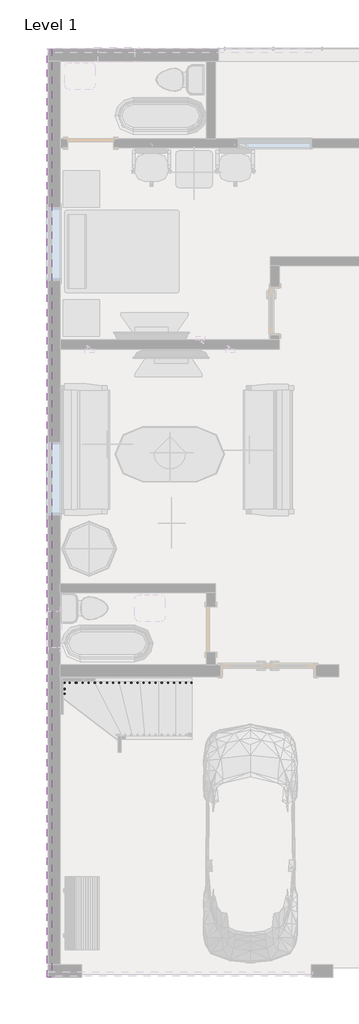
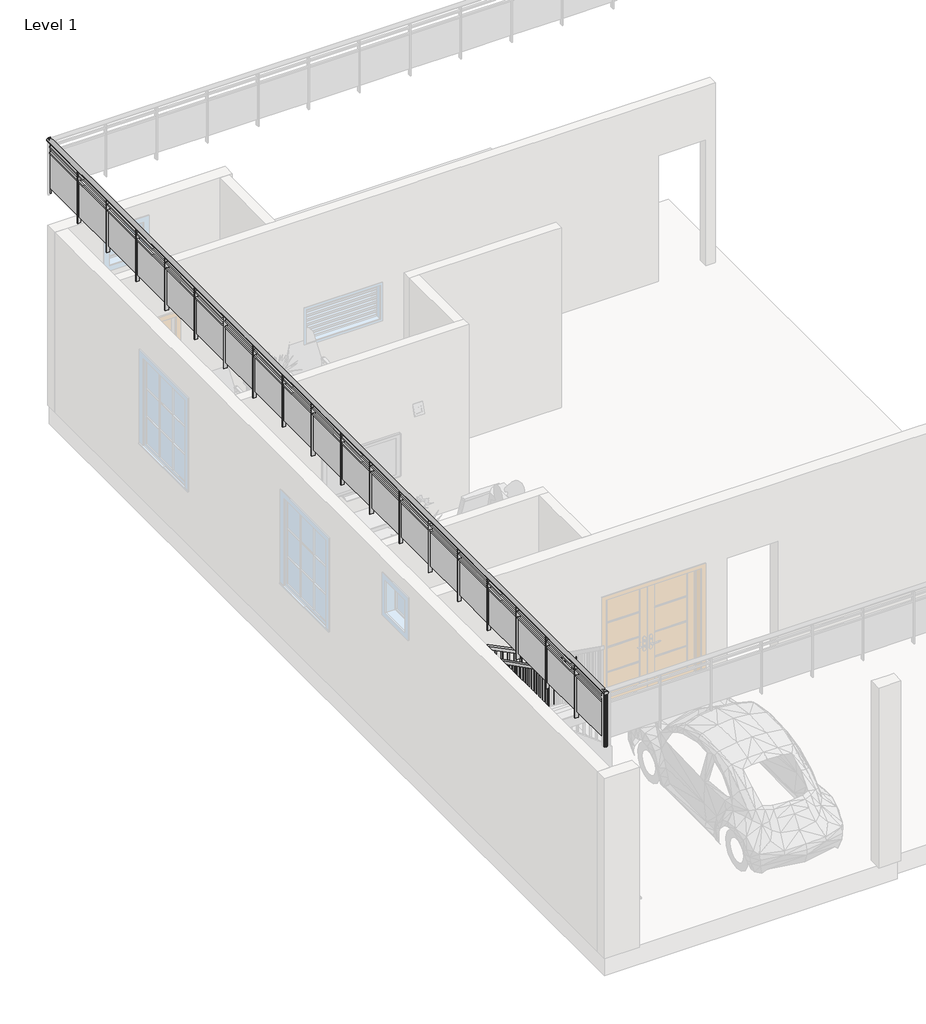
# One storey, part 3 of 5: 2 railings.
"""IFC4 building model written with IfcOpenShell, lengths in millimetres."""

from ifc_helpers import new_model, si_unit, point, frame, origin, place, context, project, spatial, polyline, ellipse_curve, trimmed, outline, extrude, faceted_brep, element, save
from ifc_brep_helpers import plane_surface, extruded_surface, advanced_brep

model = new_model("IFC4")

# Units and contexts
model_context = context("Model", 3, world=origin())
ifc_project = project(units=[si_unit("LENGTHUNIT", "METRE", prefix="MILLI")], contexts=[model_context])

# Site, building, storey
site = spatial("IfcSite", under=ifc_project)
building = spatial("IfcBuilding", under=site)
storey = spatial("IfcBuildingStorey", under=building, Name="Level 1", Elevation=0.0)

# Railings
placement = place(None, origin())
element("IfcRailing", 1, ObjectType="Glass Panel - Bottom Fill", at=placement, inside=storey, context=model_context, shape_type="SolidModel", body=[
    advanced_brep(
    [(-7235.6957152, 16067.7691167, 4495.8), (-7311.8957152, 16067.7691167, 4495.8), (-7235.6957152, 599.1691167, 4495.8), (-7311.8957152, 599.1691167, 4495.8)],
    [
        (0, 1, ellipse_curve(frame((-7273.7957152, 16067.7691167, 4495.8), z_axis=(0.0, 1.0, 0.0), x_axis=(-1.0, 0.0, 0.0)), 38.1, 28.575)),
        (1, 0, ellipse_curve(frame((-7273.7957152, 16067.7691167, 4495.8), z_axis=(0.0, 1.0, 0.0), x_axis=(-1.0, 0.0, 0.0)), 38.1, 28.575)),
        (2, 3, ellipse_curve(frame((-7273.7957152, 599.1691167, 4495.8), z_axis=(0.0, -1.0, 0.0), x_axis=(-1.0, 0.0, 0.0)), 38.1, 28.575)),
        (3, 2, ellipse_curve(frame((-7273.7957152, 599.1691167, 4495.8), z_axis=(0.0, -1.0, 0.0), x_axis=(-1.0, 0.0, 0.0)), 38.1, 28.575)),
        (0, 2),
        (3, 1),
    ],
    [
        plane_surface(frame((-7273.7957152, 16067.7691167, 4495.8), z_axis=(0.0, 1.0, 0.0), x_axis=(0.0, 0.0, -1.0))),
        plane_surface(frame((-7273.7957152, 599.1691167, 4495.8), z_axis=(0.0, -1.0, 0.0), x_axis=(0.0, 0.0, -1.0))),
        extruded_surface(trimmed(ellipse_curve(frame((-7273.7957152, 599.1691167, 4495.8), z_axis=(0.0, 1.0, 0.0), x_axis=(-1.0, 0.0, 0.0)), 38.1, 28.575), [point((-7235.6957152, 599.1691167, 4495.8))], [point((-7311.8957152, 599.1691167, 4495.8))], True, "CARTESIAN"), (0.0, 15468.599999999999, 0.0), 15468.599999999999),
        extruded_surface(trimmed(ellipse_curve(frame((-7273.7957152, 599.1691167, 4495.8), z_axis=(0.0, 1.0, 0.0), x_axis=(-1.0, 0.0, 0.0)), 38.1, 28.575), [point((-7311.8957152, 599.1691167, 4495.8))], [point((-7235.6957152, 599.1691167, 4495.8))], True, "CARTESIAN"), (0.0, 15468.599999999999, 0.0), 15468.599999999999),
    ],
    [
        (0, [[1, 2]]),
        (1, [[3, 4]]),
        (2, [[-1, 5, -4, 6]]),
        (3, [[-2, -6, -3, -5]]),
    ],
),
    extrude(outline(polyline([(-7286.4957152, 16067.7691167), (-7261.0957152, 16067.7691167), (-7261.0957152, 599.1691167), (-7286.4957152, 599.1691167), (-7286.4957152, 16067.7691167)])), frame((0.0, 0.0, 4381.5), z_axis=(0.0, 0.0, 1.0), x_axis=(1.0, 0.0, 0.0)), (0.0, 0.0, 1.0), 25.4),
    extrude(outline(polyline([(-7286.4957152, 16067.7691167), (-7261.0957152, 16067.7691167), (-7261.0957152, 599.1691167), (-7286.4957152, 599.1691167), (-7286.4957152, 16067.7691167)])), frame((0.0, 0.0, 4279.9), z_axis=(0.0, 0.0, 1.0), x_axis=(1.0, 0.0, 0.0)), (0.0, 0.0, 1.0), 25.4),
    extrude(outline(polyline([(-7299.1957152, 618.2191167), (-7248.3957152, 618.2191167), (-7248.3957152, 605.5191167), (-7299.1957152, 605.5191167), (-7299.1957152, 618.2191167)])), frame((0.0, 0.0, 3581.4), z_axis=(0.0, 0.0, 1.0), x_axis=(1.0, 0.0, 0.0)), (0.0, 0.0, 1.0), 885.6788223),
    extrude(outline(polyline([(-7267.2605581, 1424.6691167), (-7267.2605581, 611.8691167), (-7273.6105581, 611.8691167), (-7273.6105581, 1424.6691167), (-7267.2605581, 1424.6691167)])), frame((0.0, 0.0, 3683.0), z_axis=(0.0, 0.0, 1.0), x_axis=(1.0, 0.0, 0.0)), (0.0, 0.0, 1.0), 596.9),
    extrude(outline(polyline([(-7299.1957152, 1431.0191167), (-7248.3957152, 1431.0191167), (-7248.3957152, 1418.3191167), (-7299.1957152, 1418.3191167), (-7299.1957152, 1431.0191167)])), frame((0.0, 0.0, 3581.4), z_axis=(0.0, 0.0, 1.0), x_axis=(1.0, 0.0, 0.0)), (0.0, 0.0, 1.0), 885.6788223),
    extrude(outline(polyline([(-7267.2605581, 2237.4691167), (-7267.2605581, 1424.6691167), (-7273.6105581, 1424.6691167), (-7273.6105581, 2237.4691167), (-7267.2605581, 2237.4691167)])), frame((0.0, 0.0, 3683.0), z_axis=(0.0, 0.0, 1.0), x_axis=(1.0, 0.0, 0.0)), (0.0, 0.0, 1.0), 596.9),
    extrude(outline(polyline([(-7299.1957152, 2243.8191167), (-7248.3957152, 2243.8191167), (-7248.3957152, 2231.1191167), (-7299.1957152, 2231.1191167), (-7299.1957152, 2243.8191167)])), frame((0.0, 0.0, 3581.4), z_axis=(0.0, 0.0, 1.0), x_axis=(1.0, 0.0, 0.0)), (0.0, 0.0, 1.0), 885.6788223),
    extrude(outline(polyline([(-7267.2605581, 3050.2691167), (-7267.2605581, 2237.4691167), (-7273.6105581, 2237.4691167), (-7273.6105581, 3050.2691167), (-7267.2605581, 3050.2691167)])), frame((0.0, 0.0, 3683.0), z_axis=(0.0, 0.0, 1.0), x_axis=(1.0, 0.0, 0.0)), (0.0, 0.0, 1.0), 596.9),
    extrude(outline(polyline([(-7299.1957152, 3056.6191167), (-7248.3957152, 3056.6191167), (-7248.3957152, 3043.9191167), (-7299.1957152, 3043.9191167), (-7299.1957152, 3056.6191167)])), frame((0.0, 0.0, 3581.4), z_axis=(0.0, 0.0, 1.0), x_axis=(1.0, 0.0, 0.0)), (0.0, 0.0, 1.0), 885.6788223),
    extrude(outline(polyline([(-7267.2605581, 3863.0691167), (-7267.2605581, 3050.2691167), (-7273.6105581, 3050.2691167), (-7273.6105581, 3863.0691167), (-7267.2605581, 3863.0691167)])), frame((0.0, 0.0, 3683.0), z_axis=(0.0, 0.0, 1.0), x_axis=(1.0, 0.0, 0.0)), (0.0, 0.0, 1.0), 596.9),
    extrude(outline(polyline([(-7299.1957152, 3869.4191167), (-7248.3957152, 3869.4191167), (-7248.3957152, 3856.7191167), (-7299.1957152, 3856.7191167), (-7299.1957152, 3869.4191167)])), frame((0.0, 0.0, 3581.4), z_axis=(0.0, 0.0, 1.0), x_axis=(1.0, 0.0, 0.0)), (0.0, 0.0, 1.0), 885.6788223),
    extrude(outline(polyline([(-7267.2605581, 4675.8691167), (-7267.2605581, 3863.0691167), (-7273.6105581, 3863.0691167), (-7273.6105581, 4675.8691167), (-7267.2605581, 4675.8691167)])), frame((0.0, 0.0, 3683.0), z_axis=(0.0, 0.0, 1.0), x_axis=(1.0, 0.0, 0.0)), (0.0, 0.0, 1.0), 596.9),
    extrude(outline(polyline([(-7299.1957152, 4682.2191167), (-7248.3957152, 4682.2191167), (-7248.3957152, 4669.5191167), (-7299.1957152, 4669.5191167), (-7299.1957152, 4682.2191167)])), frame((0.0, 0.0, 3581.4), z_axis=(0.0, 0.0, 1.0), x_axis=(1.0, 0.0, 0.0)), (0.0, 0.0, 1.0), 885.6788223),
    extrude(outline(polyline([(-7267.2605581, 5488.6691167), (-7267.2605581, 4675.8691167), (-7273.6105581, 4675.8691167), (-7273.6105581, 5488.6691167), (-7267.2605581, 5488.6691167)])), frame((0.0, 0.0, 3683.0), z_axis=(0.0, 0.0, 1.0), x_axis=(1.0, 0.0, 0.0)), (0.0, 0.0, 1.0), 596.9),
    extrude(outline(polyline([(-7299.1957152, 5495.0191167), (-7248.3957152, 5495.0191167), (-7248.3957152, 5482.3191167), (-7299.1957152, 5482.3191167), (-7299.1957152, 5495.0191167)])), frame((0.0, 0.0, 3581.4), z_axis=(0.0, 0.0, 1.0), x_axis=(1.0, 0.0, 0.0)), (0.0, 0.0, 1.0), 885.6788223),
    extrude(outline(polyline([(-7267.2605581, 6301.4691167), (-7267.2605581, 5488.6691167), (-7273.6105581, 5488.6691167), (-7273.6105581, 6301.4691167), (-7267.2605581, 6301.4691167)])), frame((0.0, 0.0, 3683.0), z_axis=(0.0, 0.0, 1.0), x_axis=(1.0, 0.0, 0.0)), (0.0, 0.0, 1.0), 596.9),
    extrude(outline(polyline([(-7299.1957152, 6307.8191167), (-7248.3957152, 6307.8191167), (-7248.3957152, 6295.1191167), (-7299.1957152, 6295.1191167), (-7299.1957152, 6307.8191167)])), frame((0.0, 0.0, 3581.4), z_axis=(0.0, 0.0, 1.0), x_axis=(1.0, 0.0, 0.0)), (0.0, 0.0, 1.0), 885.6788223),
    extrude(outline(polyline([(-7267.2605581, 7114.2691167), (-7267.2605581, 6301.4691167), (-7273.6105581, 6301.4691167), (-7273.6105581, 7114.2691167), (-7267.2605581, 7114.2691167)])), frame((0.0, 0.0, 3683.0), z_axis=(0.0, 0.0, 1.0), x_axis=(1.0, 0.0, 0.0)), (0.0, 0.0, 1.0), 596.9),
    extrude(outline(polyline([(-7299.1957152, 7120.6191167), (-7248.3957152, 7120.6191167), (-7248.3957152, 7107.9191167), (-7299.1957152, 7107.9191167), (-7299.1957152, 7120.6191167)])), frame((0.0, 0.0, 3581.4), z_axis=(0.0, 0.0, 1.0), x_axis=(1.0, 0.0, 0.0)), (0.0, 0.0, 1.0), 885.6788223),
    extrude(outline(polyline([(-7267.2605581, 7927.0691167), (-7267.2605581, 7114.2691167), (-7273.6105581, 7114.2691167), (-7273.6105581, 7927.0691167), (-7267.2605581, 7927.0691167)])), frame((0.0, 0.0, 3683.0), z_axis=(0.0, 0.0, 1.0), x_axis=(1.0, 0.0, 0.0)), (0.0, 0.0, 1.0), 596.9),
    extrude(outline(polyline([(-7299.1957152, 7933.4191167), (-7248.3957152, 7933.4191167), (-7248.3957152, 7920.7191167), (-7299.1957152, 7920.7191167), (-7299.1957152, 7933.4191167)])), frame((0.0, 0.0, 3581.4), z_axis=(0.0, 0.0, 1.0), x_axis=(1.0, 0.0, 0.0)), (0.0, 0.0, 1.0), 885.6788223),
    extrude(outline(polyline([(-7267.2605581, 8739.8691167), (-7267.2605581, 7927.0691167), (-7273.6105581, 7927.0691167), (-7273.6105581, 8739.8691167), (-7267.2605581, 8739.8691167)])), frame((0.0, 0.0, 3683.0), z_axis=(0.0, 0.0, 1.0), x_axis=(1.0, 0.0, 0.0)), (0.0, 0.0, 1.0), 596.9),
    extrude(outline(polyline([(-7299.1957152, 8746.2191167), (-7248.3957152, 8746.2191167), (-7248.3957152, 8733.5191167), (-7299.1957152, 8733.5191167), (-7299.1957152, 8746.2191167)])), frame((0.0, 0.0, 3581.4), z_axis=(0.0, 0.0, 1.0), x_axis=(1.0, 0.0, 0.0)), (0.0, 0.0, 1.0), 885.6788223),
    extrude(outline(polyline([(-7267.2605581, 9552.6691167), (-7267.2605581, 8739.8691167), (-7273.6105581, 8739.8691167), (-7273.6105581, 9552.6691167), (-7267.2605581, 9552.6691167)])), frame((0.0, 0.0, 3683.0), z_axis=(0.0, 0.0, 1.0), x_axis=(1.0, 0.0, 0.0)), (0.0, 0.0, 1.0), 596.9),
    extrude(outline(polyline([(-7299.1957152, 9559.0191167), (-7248.3957152, 9559.0191167), (-7248.3957152, 9546.3191167), (-7299.1957152, 9546.3191167), (-7299.1957152, 9559.0191167)])), frame((0.0, 0.0, 3581.4), z_axis=(0.0, 0.0, 1.0), x_axis=(1.0, 0.0, 0.0)), (0.0, 0.0, 1.0), 885.6788223),
    extrude(outline(polyline([(-7267.2605581, 10365.4691167), (-7267.2605581, 9552.6691167), (-7273.6105581, 9552.6691167), (-7273.6105581, 10365.4691167), (-7267.2605581, 10365.4691167)])), frame((0.0, 0.0, 3683.0), z_axis=(0.0, 0.0, 1.0), x_axis=(1.0, 0.0, 0.0)), (0.0, 0.0, 1.0), 596.9),
    extrude(outline(polyline([(-7299.1957152, 10371.8191167), (-7248.3957152, 10371.8191167), (-7248.3957152, 10359.1191167), (-7299.1957152, 10359.1191167), (-7299.1957152, 10371.8191167)])), frame((0.0, 0.0, 3581.4), z_axis=(0.0, 0.0, 1.0), x_axis=(1.0, 0.0, 0.0)), (0.0, 0.0, 1.0), 885.6788223),
    extrude(outline(polyline([(-7267.2605581, 11178.2691167), (-7267.2605581, 10365.4691167), (-7273.6105581, 10365.4691167), (-7273.6105581, 11178.2691167), (-7267.2605581, 11178.2691167)])), frame((0.0, 0.0, 3683.0), z_axis=(0.0, 0.0, 1.0), x_axis=(1.0, 0.0, 0.0)), (0.0, 0.0, 1.0), 596.9),
    extrude(outline(polyline([(-7299.1957152, 11184.6191167), (-7248.3957152, 11184.6191167), (-7248.3957152, 11171.9191167), (-7299.1957152, 11171.9191167), (-7299.1957152, 11184.6191167)])), frame((0.0, 0.0, 3581.4), z_axis=(0.0, 0.0, 1.0), x_axis=(1.0, 0.0, 0.0)), (0.0, 0.0, 1.0), 885.6788223),
    extrude(outline(polyline([(-7267.2605581, 11991.0691167), (-7267.2605581, 11178.2691167), (-7273.6105581, 11178.2691167), (-7273.6105581, 11991.0691167), (-7267.2605581, 11991.0691167)])), frame((0.0, 0.0, 3683.0), z_axis=(0.0, 0.0, 1.0), x_axis=(1.0, 0.0, 0.0)), (0.0, 0.0, 1.0), 596.9),
    extrude(outline(polyline([(-7299.1957152, 11997.4191167), (-7248.3957152, 11997.4191167), (-7248.3957152, 11984.7191167), (-7299.1957152, 11984.7191167), (-7299.1957152, 11997.4191167)])), frame((0.0, 0.0, 3581.4), z_axis=(0.0, 0.0, 1.0), x_axis=(1.0, 0.0, 0.0)), (0.0, 0.0, 1.0), 885.6788223),
    extrude(outline(polyline([(-7267.2605581, 12803.8691167), (-7267.2605581, 11991.0691167), (-7273.6105581, 11991.0691167), (-7273.6105581, 12803.8691167), (-7267.2605581, 12803.8691167)])), frame((0.0, 0.0, 3683.0), z_axis=(0.0, 0.0, 1.0), x_axis=(1.0, 0.0, 0.0)), (0.0, 0.0, 1.0), 596.9),
    extrude(outline(polyline([(-7299.1957152, 12810.2191167), (-7248.3957152, 12810.2191167), (-7248.3957152, 12797.5191167), (-7299.1957152, 12797.5191167), (-7299.1957152, 12810.2191167)])), frame((0.0, 0.0, 3581.4), z_axis=(0.0, 0.0, 1.0), x_axis=(1.0, 0.0, 0.0)), (0.0, 0.0, 1.0), 885.6788223),
    extrude(outline(polyline([(-7267.2605581, 13616.6691167), (-7267.2605581, 12803.8691167), (-7273.6105581, 12803.8691167), (-7273.6105581, 13616.6691167), (-7267.2605581, 13616.6691167)])), frame((0.0, 0.0, 3683.0), z_axis=(0.0, 0.0, 1.0), x_axis=(1.0, 0.0, 0.0)), (0.0, 0.0, 1.0), 596.9),
    extrude(outline(polyline([(-7299.1957152, 13623.0191167), (-7248.3957152, 13623.0191167), (-7248.3957152, 13610.3191167), (-7299.1957152, 13610.3191167), (-7299.1957152, 13623.0191167)])), frame((0.0, 0.0, 3581.4), z_axis=(0.0, 0.0, 1.0), x_axis=(1.0, 0.0, 0.0)), (0.0, 0.0, 1.0), 885.6788223),
    extrude(outline(polyline([(-7267.2605581, 14429.4691167), (-7267.2605581, 13616.6691167), (-7273.6105581, 13616.6691167), (-7273.6105581, 14429.4691167), (-7267.2605581, 14429.4691167)])), frame((0.0, 0.0, 3683.0), z_axis=(0.0, 0.0, 1.0), x_axis=(1.0, 0.0, 0.0)), (0.0, 0.0, 1.0), 596.9),
    extrude(outline(polyline([(-7299.1957152, 14435.8191167), (-7248.3957152, 14435.8191167), (-7248.3957152, 14423.1191167), (-7299.1957152, 14423.1191167), (-7299.1957152, 14435.8191167)])), frame((0.0, 0.0, 3581.4), z_axis=(0.0, 0.0, 1.0), x_axis=(1.0, 0.0, 0.0)), (0.0, 0.0, 1.0), 885.6788223),
    extrude(outline(polyline([(-7267.2605581, 15242.2691167), (-7267.2605581, 14429.4691167), (-7273.6105581, 14429.4691167), (-7273.6105581, 15242.2691167), (-7267.2605581, 15242.2691167)])), frame((0.0, 0.0, 3683.0), z_axis=(0.0, 0.0, 1.0), x_axis=(1.0, 0.0, 0.0)), (0.0, 0.0, 1.0), 596.9),
    extrude(outline(polyline([(-7299.1957152, 15248.6191167), (-7248.3957152, 15248.6191167), (-7248.3957152, 15235.9191167), (-7299.1957152, 15235.9191167), (-7299.1957152, 15248.6191167)])), frame((0.0, 0.0, 3581.4), z_axis=(0.0, 0.0, 1.0), x_axis=(1.0, 0.0, 0.0)), (0.0, 0.0, 1.0), 885.6788223),
    extrude(outline(polyline([(-7267.2605581, 16055.0691167), (-7267.2605581, 15242.2691167), (-7273.6105581, 15242.2691167), (-7273.6105581, 16055.0691167), (-7267.2605581, 16055.0691167)])), frame((0.0, 0.0, 3683.0), z_axis=(0.0, 0.0, 1.0), x_axis=(1.0, 0.0, 0.0)), (0.0, 0.0, 1.0), 596.9),
    extrude(outline(polyline([(-7299.1957152, 16061.4191167), (-7248.3957152, 16061.4191167), (-7248.3957152, 16048.7191167), (-7299.1957152, 16048.7191167), (-7299.1957152, 16061.4191167)])), frame((0.0, 0.0, 3581.4), z_axis=(0.0, 0.0, 1.0), x_axis=(1.0, 0.0, 0.0)), (0.0, 0.0, 1.0), 885.6788223),
    extrude(outline(polyline([(-7283.3207152, 611.8691167), (-7264.2707152, 611.8691167), (-7264.2707152, 592.8191167), (-7283.3207152, 592.8191167), (-7283.3207152, 611.8691167)])), frame((0.0, 0.0, 3581.4), z_axis=(0.0, 0.0, 1.0), x_axis=(1.0, 0.0, 0.0)), (0.0, 0.0, 1.0), 885.6788223),
    extrude(outline(polyline([(-7283.3207152, 16074.1191167), (-7264.2707152, 16074.1191167), (-7264.2707152, 16055.0691167), (-7283.3207152, 16055.0691167), (-7283.3207152, 16074.1191167)])), frame((0.0, 0.0, 3581.4), z_axis=(0.0, 0.0, 1.0), x_axis=(1.0, 0.0, 0.0)), (0.0, 0.0, 1.0), 885.6788223),
])
element("IfcRailing", 2, ObjectType="Handrail - Rectangular", at=placement, inside=storey, context=model_context, shape_type="SolidModel", body=[
    faceted_brep([(-4892.6027934, 5475.9691167, 1284.0032818), (-4892.6027934, 5475.9691167, 1227.3127309), (-4892.6027934, 5526.7691167, 1227.3127309), (-4892.6027934, 5526.7691167, 1284.0032818), (-6838.0409709, 5475.9691167, 2247.6477314), (-6849.9330154, 5475.9691167, 2196.8477314), (-6849.9330154, 5526.7691167, 2196.8477314), (-6838.0409709, 5526.7691167, 2247.6477314), (-6994.3957152, 5475.9691167, 2247.6477314), (-6994.3957152, 5475.9691167, 2196.8477314), (-7045.1957152, 5526.7691167, 2196.8477314), (-7045.1957152, 5526.7691167, 2247.6477314), (-6994.3957152, 5322.5451866, 2247.6477314), (-6994.3957152, 5310.4789221, 2196.8477314), (-7045.1957152, 5310.4789221, 2196.8477314), (-7045.1957152, 5322.5451866, 2247.6477314), (-6994.3957152, 2646.197182, 3595.0649553), (-7045.1957152, 2646.197182, 3595.0649553), (-7045.1957152, 2646.197182, 3538.1901501), (-6994.3957152, 2646.197182, 3538.1901501)], [[[0, 1, 2, 3]], [[1, 0, 4, 5]], [[2, 1, 5, 6]], [[3, 2, 6, 7]], [[0, 3, 7, 4]], [[5, 4, 8, 9]], [[6, 5, 9, 10]], [[7, 6, 10, 11]], [[4, 7, 11, 8]], [[9, 8, 12, 13]], [[10, 9, 13, 14]], [[11, 10, 14, 15]], [[8, 11, 15, 12]], [[16, 17, 18, 19]], [[13, 12, 16, 19]], [[14, 13, 19, 18]], [[15, 14, 18, 17]], [[12, 15, 17, 16]]]),
    extrude(outline(polyline([(2671.4201866, 3525.4915359), (2690.4701866, 3515.9007435), (2690.4701866, 2540.0), (2671.4201866, 2540.0), (2671.4201866, 3525.4915359)])), frame((-7029.3207152, 0.0, 0.0), z_axis=(1.0, 0.0, 0.0), x_axis=(0.0, 1.0, 0.0)), (0.0, 0.0, 1.0), 19.05),
    extrude(outline(polyline([(2773.0201866, 3474.3406431), (2792.0701866, 3464.7498507), (2792.0701866, 2540.0), (2773.0201866, 2540.0), (2773.0201866, 3474.3406431)])), frame((-7029.3207152, 0.0, 0.0), z_axis=(1.0, 0.0, 0.0), x_axis=(0.0, 1.0, 0.0)), (0.0, 0.0, 1.0), 19.05),
    extrude(outline(polyline([(2874.6201866, 3423.1897503), (2893.6701866, 3413.5989579), (2893.6701866, 2540.0), (2874.6201866, 2540.0), (2874.6201866, 3423.1897503)])), frame((-7029.3207152, 0.0, 0.0), z_axis=(1.0, 0.0, 0.0), x_axis=(0.0, 1.0, 0.0)), (0.0, 0.0, 1.0), 19.05),
    extrude(outline(polyline([(2976.2201866, 3372.0388574), (2995.2701866, 3362.448065), (2995.2701866, 2370.6666667), (2976.2201866, 2370.6666667), (2976.2201866, 3372.0388574)])), frame((-7029.3207152, 0.0, 0.0), z_axis=(1.0, 0.0, 0.0), x_axis=(0.0, 1.0, 0.0)), (0.0, 0.0, 1.0), 19.05),
    extrude(outline(polyline([(3077.8201866, 3320.8879646), (3096.8701866, 3311.2971722), (3096.8701866, 2370.6666667), (3077.8201866, 2370.6666667), (3077.8201866, 3320.8879646)])), frame((-7029.3207152, 0.0, 0.0), z_axis=(1.0, 0.0, 0.0), x_axis=(0.0, 1.0, 0.0)), (0.0, 0.0, 1.0), 19.05),
    extrude(outline(polyline([(3179.4201866, 3269.7370718), (3198.4701866, 3260.1462794), (3198.4701866, 2370.6666667), (3179.4201866, 2370.6666667), (3179.4201866, 3269.7370718)])), frame((-7029.3207152, 0.0, 0.0), z_axis=(1.0, 0.0, 0.0), x_axis=(0.0, 1.0, 0.0)), (0.0, 0.0, 1.0), 19.05),
    extrude(outline(polyline([(3281.0201866, 3218.586179), (3300.0701866, 3208.9953866), (3300.0701866, 2201.3333333), (3281.0201866, 2201.3333333), (3281.0201866, 3218.586179)])), frame((-7029.3207152, 0.0, 0.0), z_axis=(1.0, 0.0, 0.0), x_axis=(0.0, 1.0, 0.0)), (0.0, 0.0, 1.0), 19.05),
    extrude(outline(polyline([(3382.6201866, 3167.4352861), (3401.6701866, 3157.8444937), (3401.6701866, 2201.3333333), (3382.6201866, 2201.3333333), (3382.6201866, 3167.4352861)])), frame((-7029.3207152, 0.0, 0.0), z_axis=(1.0, 0.0, 0.0), x_axis=(0.0, 1.0, 0.0)), (0.0, 0.0, 1.0), 19.05),
    extrude(outline(polyline([(3484.2201866, 3116.2843933), (3503.2701866, 3106.6936009), (3503.2701866, 2201.3333333), (3484.2201866, 2201.3333333), (3484.2201866, 3116.2843933)])), frame((-7029.3207152, 0.0, 0.0), z_axis=(1.0, 0.0, 0.0), x_axis=(0.0, 1.0, 0.0)), (0.0, 0.0, 1.0), 19.05),
    extrude(outline(polyline([(3585.8201866, 3065.1335005), (3604.8701866, 3055.5427081), (3604.8701866, 2032.0), (3585.8201866, 2032.0), (3585.8201866, 3065.1335005)])), frame((-7029.3207152, 0.0, 0.0), z_axis=(1.0, 0.0, 0.0), x_axis=(0.0, 1.0, 0.0)), (0.0, 0.0, 1.0), 19.05),
    extrude(outline(polyline([(3687.4201866, 3013.9826077), (3706.4701866, 3004.3918153), (3706.4701866, 2032.0), (3687.4201866, 2032.0), (3687.4201866, 3013.9826077)])), frame((-7029.3207152, 0.0, 0.0), z_axis=(1.0, 0.0, 0.0), x_axis=(0.0, 1.0, 0.0)), (0.0, 0.0, 1.0), 19.05),
    extrude(outline(polyline([(3789.0201866, 2962.8317148), (3808.0701866, 2953.2409224), (3808.0701866, 2032.0), (3789.0201866, 2032.0), (3789.0201866, 2962.8317148)])), frame((-7029.3207152, 0.0, 0.0), z_axis=(1.0, 0.0, 0.0), x_axis=(0.0, 1.0, 0.0)), (0.0, 0.0, 1.0), 19.05),
    extrude(outline(polyline([(3890.6201866, 2911.680822), (3909.6701866, 2902.0900296), (3909.6701866, 1862.6666667), (3890.6201866, 1862.6666667), (3890.6201866, 2911.680822)])), frame((-7029.3207152, 0.0, 0.0), z_axis=(1.0, 0.0, 0.0), x_axis=(0.0, 1.0, 0.0)), (0.0, 0.0, 1.0), 19.05),
    extrude(outline(polyline([(3992.2201866, 2860.5299292), (4011.2701866, 2850.9391368), (4011.2701866, 1862.6666667), (3992.2201866, 1862.6666667), (3992.2201866, 2860.5299292)])), frame((-7029.3207152, 0.0, 0.0), z_axis=(1.0, 0.0, 0.0), x_axis=(0.0, 1.0, 0.0)), (0.0, 0.0, 1.0), 19.05),
    extrude(outline(polyline([(4093.8201866, 2809.3790364), (4112.8701866, 2799.788244), (4112.8701866, 1862.6666667), (4093.8201866, 1862.6666667), (4093.8201866, 2809.3790364)])), frame((-7029.3207152, 0.0, 0.0), z_axis=(1.0, 0.0, 0.0), x_axis=(0.0, 1.0, 0.0)), (0.0, 0.0, 1.0), 19.05),
    extrude(outline(polyline([(4195.4201866, 2758.2281435), (4214.4701866, 2748.6373511), (4214.4701866, 1693.3333333), (4195.4201866, 1693.3333333), (4195.4201866, 2758.2281435)])), frame((-7029.3207152, 0.0, 0.0), z_axis=(1.0, 0.0, 0.0), x_axis=(0.0, 1.0, 0.0)), (0.0, 0.0, 1.0), 19.05),
    extrude(outline(polyline([(4297.0201866, 2707.0772507), (4316.0701866, 2697.4864583), (4316.0701866, 1693.3333333), (4297.0201866, 1693.3333333), (4297.0201866, 2707.0772507)])), frame((-7029.3207152, 0.0, 0.0), z_axis=(1.0, 0.0, 0.0), x_axis=(0.0, 1.0, 0.0)), (0.0, 0.0, 1.0), 19.05),
    extrude(outline(polyline([(4398.6201866, 2655.9263579), (4417.6701866, 2646.3355655), (4417.6701866, 1693.3333333), (4398.6201866, 1693.3333333), (4398.6201866, 2655.9263579)])), frame((-7029.3207152, 0.0, 0.0), z_axis=(1.0, 0.0, 0.0), x_axis=(0.0, 1.0, 0.0)), (0.0, 0.0, 1.0), 19.05),
    extrude(outline(polyline([(4500.2201866, 2604.7754651), (4519.2701866, 2595.1846727), (4519.2701866, 1524.0), (4500.2201866, 1524.0), (4500.2201866, 2604.7754651)])), frame((-7029.3207152, 0.0, 0.0), z_axis=(1.0, 0.0, 0.0), x_axis=(0.0, 1.0, 0.0)), (0.0, 0.0, 1.0), 19.05),
    extrude(outline(polyline([(4601.8201866, 2553.6245722), (4620.8701866, 2544.0337798), (4620.8701866, 1524.0), (4601.8201866, 1524.0), (4601.8201866, 2553.6245722)])), frame((-7029.3207152, 0.0, 0.0), z_axis=(1.0, 0.0, 0.0), x_axis=(0.0, 1.0, 0.0)), (0.0, 0.0, 1.0), 19.05),
    extrude(outline(polyline([(4703.4201866, 2502.4736794), (4722.4701866, 2492.882887), (4722.4701866, 1524.0), (4703.4201866, 1524.0), (4703.4201866, 2502.4736794)])), frame((-7029.3207152, 0.0, 0.0), z_axis=(1.0, 0.0, 0.0), x_axis=(0.0, 1.0, 0.0)), (0.0, 0.0, 1.0), 19.05),
    extrude(outline(polyline([(4805.0201866, 2451.3227866), (4824.0701866, 2441.7319942), (4824.0701866, 1354.6666667), (4805.0201866, 1354.6666667), (4805.0201866, 2451.3227866)])), frame((-7029.3207152, 0.0, 0.0), z_axis=(1.0, 0.0, 0.0), x_axis=(0.0, 1.0, 0.0)), (0.0, 0.0, 1.0), 19.05),
    extrude(outline(polyline([(4906.6201866, 2400.1718938), (4925.6701866, 2390.5811014), (4925.6701866, 1354.6666667), (4906.6201866, 1354.6666667), (4906.6201866, 2400.1718938)])), frame((-7029.3207152, 0.0, 0.0), z_axis=(1.0, 0.0, 0.0), x_axis=(0.0, 1.0, 0.0)), (0.0, 0.0, 1.0), 19.05),
    extrude(outline(polyline([(5008.2201866, 2349.0210009), (5027.2701866, 2339.4302085), (5027.2701866, 1354.6666667), (5008.2201866, 1354.6666667), (5008.2201866, 2349.0210009)])), frame((-7029.3207152, 0.0, 0.0), z_axis=(1.0, 0.0, 0.0), x_axis=(0.0, 1.0, 0.0)), (0.0, 0.0, 1.0), 19.05),
    extrude(outline(polyline([(5109.8201866, 2297.8701081), (5128.8701866, 2288.2793157), (5128.8701866, 1354.6666667), (5109.8201866, 1354.6666667), (5109.8201866, 2297.8701081)])), frame((-7029.3207152, 0.0, 0.0), z_axis=(1.0, 0.0, 0.0), x_axis=(0.0, 1.0, 0.0)), (0.0, 0.0, 1.0), 19.05),
    extrude(outline(polyline([(5211.4201866, 2246.7192153), (5230.4701866, 2237.1284229), (5230.4701866, 1354.6666667), (5211.4201866, 1354.6666667), (5211.4201866, 2246.7192153)])), frame((-7029.3207152, 0.0, 0.0), z_axis=(1.0, 0.0, 0.0), x_axis=(0.0, 1.0, 0.0)), (0.0, 0.0, 1.0), 19.05),
    extrude(outline(polyline([(-7029.3207152, 5409.2941167), (-7010.2707152, 5409.2941167), (-7010.2707152, 5390.2441167), (-7029.3207152, 5390.2441167), (-7029.3207152, 5409.2941167)])), frame((0.0, 0.0, 1185.3333333), z_axis=(0.0, 0.0, 1.0), x_axis=(1.0, 0.0, 0.0)), (0.0, 0.0, 1.0), 1011.5143981),
    extrude(outline(polyline([(-6930.1159709, 5510.8941167), (-6930.1159709, 5491.8441167), (-6949.1659709, 5491.8441167), (-6949.1659709, 5510.8941167), (-6930.1159709, 5510.8941167)])), frame((0.0, 0.0, 1185.3333333), z_axis=(0.0, 0.0, 1.0), x_axis=(1.0, 0.0, 0.0)), (0.0, 0.0, 1.0), 1011.5143981),
    extrude(outline(polyline([(2178.7901685, -6813.4777934), (2188.2263084, -6832.5277934), (1185.3333333, -6832.5277934), (1185.3333333, -6813.4777934), (2178.7901685, -6813.4777934)])), frame((0.0, 5491.8441167, 0.0), z_axis=(0.0, 1.0, 0.0), x_axis=(0.0, 0.0, 1.0)), (0.0, 0.0, 1.0), 19.05),
    extrude(outline(polyline([(2128.4640891, -6711.8777934), (2137.900229, -6730.9277934), (1185.3333333, -6730.9277934), (1185.3333333, -6711.8777934), (2128.4640891, -6711.8777934)])), frame((0.0, 5491.8441167, 0.0), z_axis=(0.0, 1.0, 0.0), x_axis=(0.0, 0.0, 1.0)), (0.0, 0.0, 1.0), 19.05),
    extrude(outline(polyline([(2078.1380098, -6610.2777934), (2087.5741497, -6629.3277934), (1185.3333333, -6629.3277934), (1185.3333333, -6610.2777934), (2078.1380098, -6610.2777934)])), frame((0.0, 5491.8441167, 0.0), z_axis=(0.0, 1.0, 0.0), x_axis=(0.0, 0.0, 1.0)), (0.0, 0.0, 1.0), 19.05),
    extrude(outline(polyline([(2027.8226942, -6508.6777934), (2037.2889627, -6527.7277934), (1016.0, -6527.7277934), (1016.0, -6508.6777934), (2027.8226942, -6508.6777934)])), frame((0.0, 5491.8441167, 0.0), z_axis=(0.0, 1.0, 0.0), x_axis=(0.0, 0.0, 1.0)), (0.0, 0.0, 1.0), 19.05),
    extrude(outline(polyline([(1977.4858511, -6407.0777934), (1986.921991, -6426.1277934), (1016.0, -6426.1277934), (1016.0, -6407.0777934), (1977.4858511, -6407.0777934)])), frame((0.0, 5491.8441167, 0.0), z_axis=(0.0, 1.0, 0.0), x_axis=(0.0, 0.0, 1.0)), (0.0, 0.0, 1.0), 19.05),
    extrude(outline(polyline([(1927.1597718, -6305.4777934), (1936.5959116, -6324.5277934), (1016.0, -6324.5277934), (1016.0, -6305.4777934), (1927.1597718, -6305.4777934)])), frame((0.0, 5491.8441167, 0.0), z_axis=(0.0, 1.0, 0.0), x_axis=(0.0, 0.0, 1.0)), (0.0, 0.0, 1.0), 19.05),
    extrude(outline(polyline([(1876.8336924, -6203.8777934), (1886.2698323, -6222.9277934), (1016.0, -6222.9277934), (1016.0, -6203.8777934), (1876.8336924, -6203.8777934)])), frame((0.0, 5491.8441167, 0.0), z_axis=(0.0, 1.0, 0.0), x_axis=(0.0, 0.0, 1.0)), (0.0, 0.0, 1.0), 19.05),
    extrude(outline(polyline([(1826.5076131, -6102.2777934), (1835.9437529, -6121.3277934), (846.6666667, -6121.3277934), (846.6666667, -6102.2777934), (1826.5076131, -6102.2777934)])), frame((0.0, 5491.8441167, 0.0), z_axis=(0.0, 1.0, 0.0), x_axis=(0.0, 0.0, 1.0)), (0.0, 0.0, 1.0), 19.05),
    extrude(outline(polyline([(1776.1815337, -6000.6777934), (1785.6176736, -6019.7277934), (846.6666667, -6019.7277934), (846.6666667, -6000.6777934), (1776.1815337, -6000.6777934)])), frame((0.0, 5491.8441167, 0.0), z_axis=(0.0, 1.0, 0.0), x_axis=(0.0, 0.0, 1.0)), (0.0, 0.0, 1.0), 19.05),
    extrude(outline(polyline([(1725.8554544, -5899.0777934), (1735.2915943, -5918.1277934), (846.6666667, -5918.1277934), (846.6666667, -5899.0777934), (1725.8554544, -5899.0777934)])), frame((0.0, 5491.8441167, 0.0), z_axis=(0.0, 1.0, 0.0), x_axis=(0.0, 0.0, 1.0)), (0.0, 0.0, 1.0), 19.05),
    extrude(outline(polyline([(1675.529375, -5797.4777934), (1684.9655149, -5816.5277934), (846.6666667, -5816.5277934), (846.6666667, -5797.4777934), (1675.529375, -5797.4777934)])), frame((0.0, 5491.8441167, 0.0), z_axis=(0.0, 1.0, 0.0), x_axis=(0.0, 0.0, 1.0)), (0.0, 0.0, 1.0), 19.05),
    extrude(outline(polyline([(1625.2032957, -5695.8777934), (1634.6394356, -5714.9277934), (677.3333333, -5714.9277934), (677.3333333, -5695.8777934), (1625.2032957, -5695.8777934)])), frame((0.0, 5491.8441167, 0.0), z_axis=(0.0, 1.0, 0.0), x_axis=(0.0, 0.0, 1.0)), (0.0, 0.0, 1.0), 19.05),
    extrude(outline(polyline([(1574.8772163, -5594.2777934), (1584.3133562, -5613.3277934), (677.3333333, -5613.3277934), (677.3333333, -5594.2777934), (1574.8772163, -5594.2777934)])), frame((0.0, 5491.8441167, 0.0), z_axis=(0.0, 1.0, 0.0), x_axis=(0.0, 0.0, 1.0)), (0.0, 0.0, 1.0), 19.05),
    extrude(outline(polyline([(1524.551137, -5492.6777934), (1533.9872769, -5511.7277934), (677.3333333, -5511.7277934), (677.3333333, -5492.6777934), (1524.551137, -5492.6777934)])), frame((0.0, 5491.8441167, 0.0), z_axis=(0.0, 1.0, 0.0), x_axis=(0.0, 0.0, 1.0)), (0.0, 0.0, 1.0), 19.05),
    extrude(outline(polyline([(1474.2250577, -5391.0777934), (1483.6611975, -5410.1277934), (508.0, -5410.1277934), (508.0, -5391.0777934), (1474.2250577, -5391.0777934)])), frame((0.0, 5491.8441167, 0.0), z_axis=(0.0, 1.0, 0.0), x_axis=(0.0, 0.0, 1.0)), (0.0, 0.0, 1.0), 19.05),
    extrude(outline(polyline([(1423.8989783, -5289.4777934), (1433.3351182, -5308.5277934), (508.0, -5308.5277934), (508.0, -5289.4777934), (1423.8989783, -5289.4777934)])), frame((0.0, 5491.8441167, 0.0), z_axis=(0.0, 1.0, 0.0), x_axis=(0.0, 0.0, 1.0)), (0.0, 0.0, 1.0), 19.05),
    extrude(outline(polyline([(1373.572899, -5187.8777934), (1383.0090388, -5206.9277934), (508.0, -5206.9277934), (508.0, -5187.8777934), (1373.572899, -5187.8777934)])), frame((0.0, 5491.8441167, 0.0), z_axis=(0.0, 1.0, 0.0), x_axis=(0.0, 0.0, 1.0)), (0.0, 0.0, 1.0), 19.05),
    extrude(outline(polyline([(1323.2468196, -5086.2777934), (1332.6829595, -5105.3277934), (338.6666667, -5105.3277934), (338.6666667, -5086.2777934), (1323.2468196, -5086.2777934)])), frame((0.0, 5491.8441167, 0.0), z_axis=(0.0, 1.0, 0.0), x_axis=(0.0, 0.0, 1.0)), (0.0, 0.0, 1.0), 19.05),
    extrude(outline(polyline([(1272.9207403, -4984.6777934), (1282.3568801, -5003.7277934), (338.6666667, -5003.7277934), (338.6666667, -4984.6777934), (1272.9207403, -4984.6777934)])), frame((0.0, 5491.8441167, 0.0), z_axis=(0.0, 1.0, 0.0), x_axis=(0.0, 0.0, 1.0)), (0.0, 0.0, 1.0), 19.05),
    extrude(outline(polyline([(-7029.3207152, 5332.0701866), (-7010.2707152, 5332.0701866), (-7010.2707152, 5313.0201866), (-7029.3207152, 5313.0201866), (-7029.3207152, 5332.0701866)])), frame((0.0, 0.0, 1185.3333333), z_axis=(0.0, 0.0, 1.0), x_axis=(1.0, 0.0, 0.0)), (0.0, 0.0, 1.0), 1011.5143981),
    extrude(outline(polyline([(-7010.2707152, 5510.8941167), (-7010.2707152, 5491.8441167), (-7029.3207152, 5491.8441167), (-7029.3207152, 5510.8941167), (-7010.2707152, 5510.8941167)])), frame((0.0, 0.0, 1185.3333333), z_axis=(0.0, 0.0, 1.0), x_axis=(1.0, 0.0, 0.0)), (0.0, 0.0, 1.0), 1011.5143981),
    extrude(outline(polyline([(2186.2391105, -6828.5159709), (2195.6752504, -6847.5659709), (1185.3333333, -6847.5659709), (1185.3333333, -6828.5159709), (2186.2391105, -6828.5159709)])), frame((0.0, 5491.8441167, 0.0), z_axis=(0.0, 1.0, 0.0), x_axis=(0.0, 0.0, 1.0)), (0.0, 0.0, 1.0), 19.05),
    extrude(outline(polyline([(2646.197182, 3538.1901501), (2665.247182, 3528.5993577), (2665.247182, 2540.0), (2646.197182, 2540.0), (2646.197182, 3538.1901501)])), frame((-7029.3207152, 0.0, 0.0), z_axis=(1.0, 0.0, 0.0), x_axis=(0.0, 1.0, 0.0)), (0.0, 0.0, 1.0), 19.05),
    extrude(outline(polyline([(1227.3127309, -4892.6027934), (1236.7488707, -4911.6527934), (338.6666667, -4911.6527934), (338.6666667, -4892.6027934), (1227.3127309, -4892.6027934)])), frame((0.0, 5491.8441167, 0.0), z_axis=(0.0, 1.0, 0.0), x_axis=(0.0, 0.0, 1.0)), (0.0, 0.0, 1.0), 19.05),
])

save(model, "model.ifc")

# Revit data of these elements
# Type "Glass Panel - Bottom Fill"
#   Assembly Code = "C2010400"
#   built-in parameter 1008612 = 0.0416667 (stored number, unit not read)
#   built-in parameter 1008611 = 0.0416667 (stored number, unit not read)
#   built-in parameter 1008609 = 0.333333 (stored number, unit not read)
#   built-in parameter 1008604 = 0.166667 (stored number, unit not read)
#   built-in parameter 1008603 = 0.166667 (stored number, unit not read)
#   Railing Height = 3' - 0"
#   built-in parameter 1008630 = 2
#   built-in parameter 1008610 = 2
#   built-in parameter 1008618 = Baluster - Square : 3/4"
# Type "Handrail - Rectangular"
#   Assembly Code = "C2010400"
#   built-in parameter 1008612 = 0.0416667 (stored number, unit not read)
#   built-in parameter 1008611 = 0.0416667 (stored number, unit not read)
#   built-in parameter 1008609 = 0.333333 (stored number, unit not read)
#   built-in parameter 1008604 = 0.166667 (stored number, unit not read)
#   built-in parameter 1008603 = 0.166667 (stored number, unit not read)
#   Railing Height = 3' - 0"
#   built-in parameter 1008630 = 2
#   built-in parameter 1008610 = 2
#   built-in parameter 1008618 = Baluster - Square : 3/4"
# Element 1 (IfcRailing, "Glass Panel - Bottom Fill")
#   built-in parameter 1008621 = 11.75 (stored number, unit not read)
#   Phase Created = New Construction
#   Materials on its faces: "Glass"
# Element 2 (IfcRailing, "Handrail - Rectangular")
#   Phase Created = New Construction
# Materials
#   "Glass": class "Glass", colour RGB 0 128 192, transparency 0.75, Description = "Soda Lime Glass", Cost = 0
